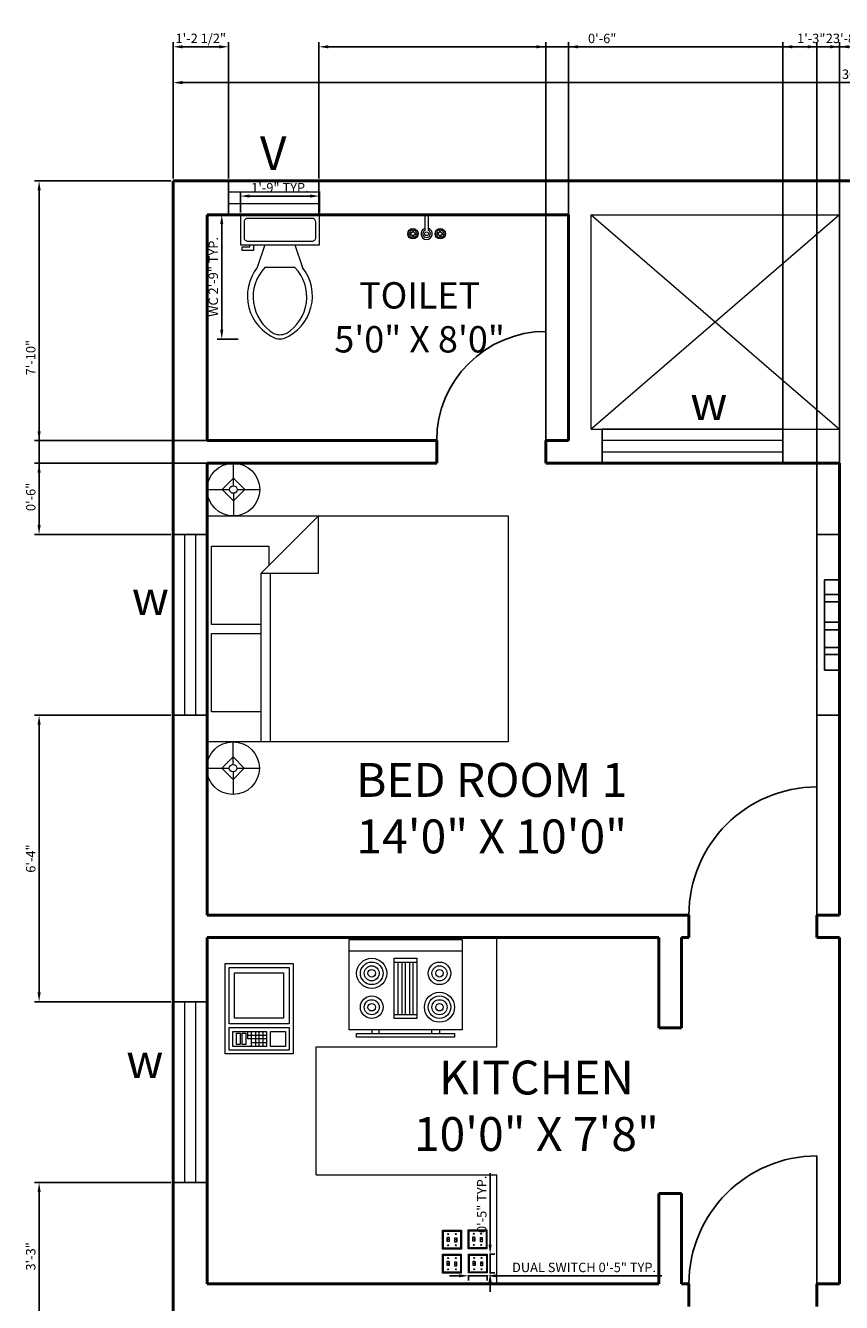
# Model space of a CAD drawing. Units: inches. Extents: x 3688 to 4628, y 1593 to 2337.
# Tile 3 of 7: x 3690 to 3907, y 1997 to 2337. Entities that reach past the tile are written whole.
import ezdxf

# ---------------------------------------------------------------- set-up
doc = ezdxf.new("R2010")
doc.units = ezdxf.units.IN
for name, color, linetype, lineweight in [('A-ANNO-DIMS', 2, 'Continuous', 18), ('A-ANNO-TEXT', 7, 'Continuous', 18), ('A-AREA-IDEN', 7, 'Continuous', 25), ('A-DOOR', 4, 'Continuous', 25), ('A-EQPM', 8, 'Continuous', 18), ('A-FLOR-FIXT', 8, 'Continuous', 18), ('A-FLOR-SHFT', 8, 'Continuous', 18), ('A-FURN', 8, 'Continuous', 18), ('A-GLAZ', 4, 'Continuous', 25), ('A-WALL', 7, 'Continuous', 50), ('E-LITE', 6, 'Continuous', 18)]:
    doc.layers.add(name, color=color, linetype=linetype, lineweight=lineweight)
doc.styles.get("Standard").update_dxf_attribs({"font": 'arial.ttf'})
doc.dimstyles.new('ISO-25', dxfattribs={"dimtxt": 2.5, "dimasz": 2.5, "dimexe": 1.25, "dimexo": 0.625, "dimtad": 1, "dimdec": 0, "dimlunit": 3, "dimtxsty": 'Standard', "dimcen": 2.5, "dimadec": 0, "dimazin": 0, "dimtfac": 1, "dimtdec": 0, "dimtmove": 0, "dimatfit": 3, "dimfxl": 1, "dimarcsym": 0})

# ---------------------------------------------------------------- blocks, each defined once
blk = doc.blocks.new('Toilet - top')
for p, q in [((9.5, -6), (9.5, -2)), ((-10, -8.5), (-8, -8.5)), ((-10, -9.5), (-10, -8.5)), ((-7, -9.5), (-10, -9.5)), ((-8, -8.5), (-8, -8)), ((-7, -8), (-7, -9.5)), ((-4, -8), (-6, -14)), ((4, -8), (6, -14)), ((4, -14), (-4, -14))]:
    blk.add_line(p, q)
blk.add_lwpolyline([(10.5, -8), (10.5, 0), (-10.5, 0), (-10.5, -8)], close=True)
for points in [[(-9.5, -2), (-9.5, -6)], [(8.5, -1), (-8.5, -1)], [(-8.5, -7), (8.5, -7)]]:
    blk.add_lwpolyline(points)
for centre, radius, start, end in [((-8.62, -1.88), 0.884, 81.8699, 188.1301), ((8.62, -1.88), 0.884, 351.8699, 98.1301), ((-8.62, -6.12), 0.884, 171.8699, 278.1301), ((8.62, -6.12), 0.884, 261.8699, 8.1301), ((3.52, -21.58), 12.17, 141.4691, 247.9714), ((4.2, -21.82), 11.33, 136.3677, 238.9468), ((-3.52, -21.58), 12.17, 292.0284, 38.5307), ((-4.2, -21.82), 11.33, 301.053, 43.6321), ((0, -27.88), 4, 245.7318, 294.2682), ((0, -29), 4, 254.8605, 285.1395)]:
    blk.add_arc(centre, radius, start, end)
blk = doc.blocks.new('Bed - Queen')
for p, q in [((0, -80.00003), (0, 0)), ((0, 0), (59.99999, 0)), ((59.99999, 0), (59.99999, -80.00003)), ((7.99999, -1.2), (28.79998, -1.2)), ((7.99999, -14.4), (7.99999, -1.2)), ((28.79998, -1.2), (28.79998, -14.4)), ((31.19999, -1.2), (51.99999, -1.2)), ((31.19999, -14.4), (31.19999, -1.2)), ((51.99999, -1.2), (51.99999, -16.4)), ((0, -14.4), (44.8, -14.4)), ((44.8, -16.8), (0, -16.8)), ((59.99999, -29.6), (44.8, -14.4)), ((44.8, -14.4), (44.8, -29.6)), ((51.99999, -16.4), (46.79936, -16.4)), ((44.8, -29.6), (59.99999, -29.6)), ((59.99999, -80.00003), (0, -80.00003))]:
    blk.add_line(p, q)
blk = doc.blocks.new('Lamp - Table')
for p, q in [((0, 7), (0, 1)), ((-1, 0), (-7, 0)), ((0, 3), (-3, 0)), ((-3, 0), (0, -3)), ((3, 0), (0, 3)), ((0, -3), (3, 0)), ((1, 0), (7, 0)), ((0, -1), (0, -7))]:
    blk.add_line(p, q)
for radius in [7, 1]:
    blk.add_circle((0, 0), radius)
blk = doc.blocks.new('Range-Oven - 30 in top')
for p, q in [((0, -3), (30, -3)), ((12, -6), (18, -6)), ((13, -20), (13, -6)), ((14, -6), (14, -20)), ((15, -20), (15, -6)), ((16, -6), (16, -20)), ((17, -20), (17, -6)), ((18, -20), (12, -20)), ((6, -24), (6, -25)), ((8, -25), (8, -24)), ((22, -25), (22, -24)), ((24, -24), (24, -25))]:
    blk.add_line(p, q)
for points in [[(0, -24), (0, 0), (30, 0), (30, -24)], [(12, -21), (12, -5), (18, -5), (18, -21)], [(2, -26), (2, -25), (28, -25), (28, -26)]]:
    blk.add_lwpolyline(points, close=True)
for centre, radius in [((6, -9), 4), ((6, -9), 3), ((24, -9), 3), ((6, -9), 2), ((6, -9), 1), ((24, -9), 2), ((24, -9), 1), ((6, -18), 3), ((6, -18), 2), ((24, -18), 4), ((24, -18), 3), ((24, -18), 2), ((6, -18), 1), ((24, -18), 1)]:
    blk.add_circle(centre, radius)
blk = doc.blocks.new('Microwave')
for p, q in [((19, 7), (19, 11)), ((20, 11), (20, 7)), ((21, 7), (21, 11)), ((18, 10), (22, 10)), ((22, 9), (18, 9)), ((18, 8), (22, 8)), ((22, 7), (18, 7)), ((19, 6), (19, 7)), ((20, 7), (20, 6)), ((20, 6), (18, 6))]:
    blk.add_line(p, q)
for points in [[(0, 0), (0, 18), (24, 18), (24, 0)], [(1, 1), (1, 17), (16, 17), (16, 1)], [(17, 1), (17, 17), (23, 17), (23, 1)], [(2.5, 2.5), (2.5, 15.5), (14.5, 15.5), (14.5, 2.5)], [(18, 12), (18, 16), (22, 16), (22, 12)], [(18, 2), (18, 11), (22, 11), (22, 2)], [(18.5, 4.5), (18.5, 5.5), (21.5, 5.5), (21.5, 4.5)], [(18.5, 3), (18.5, 4), (21.5, 4), (21.5, 3)]]:
    blk.add_lwpolyline(points, close=True)
blk = doc.blocks.new('Light Switch - Dual')
for p, q in [((-2.25, 4.75), (-2.5, 5)), ((-2.25, 4.75), (2.25, 4.75)), ((-2.25, 0.25), (-2.25, 4.75)), ((-0.875, 4), (-1.125, 4)), ((0.875, 4), (1.125, 4)), ((2.25, 4.75), (2.5, 5)), ((2.25, 4.75), (2.25, 0.25)), ((-2.25, 0.25), (-2.5, 0)), ((2.25, 0.25), (-2.25, 0.25)), ((-0.7854, 2.5), (-1.2183, 2.5)), ((-0.875, 1), (-1.125, 1)), ((0.7854, 2.5), (1.2182, 2.5)), ((0.875, 1), (1.125, 1)), ((2.25, 0.25), (2.5, 0))]:
    blk.add_line(p, q)
for points in [[(-2.5, 0), (-2.5, 5), (2.5, 5), (2.5, 0)], [(-0.78, 3.125), (-0.78, 2), (-1.22, 2), (-1.22, 3.125)], [(0.78, 1.875), (0.78, 3), (1.22, 3), (1.22, 1.875)]]:
    blk.add_lwpolyline(points, close=True)
for points in [[(-0.7818, 3), (-0.75, 3), (-0.75, 2), (-1.25, 2), (-1.25, 3), (-1.2219, 3)], [(0.7817, 2), (0.75, 2), (0.75, 3), (1.25, 3), (1.25, 2), (1.2219, 2)]]:
    blk.add_lwpolyline(points)
for centre in [(-1, 4), (1, 4), (-1, 1), (1, 1)]:
    blk.add_circle(centre, 0.125)
blk = doc.blocks.new('Faucet - Bathroom top')
for p, q in [((-4.107, 0.125), (-4.375, 0.125)), ((-3.75, 0.4788), (-3.75, 0.75)), ((-3.5, 0.482), (-3.5, 0.75)), ((-3.1461, 0.125), (-2.875, 0.125)), ((3.143, 0.125), (2.875, 0.125)), ((3.5, 0.4788), (3.5, 0.75)), ((3.75, 0.482), (3.75, 0.75)), ((4.1039, 0.125), (4.375, 0.125)), ((-4.1039, -0.125), (-4.375, -0.125)), ((-3.75, -0.4821), (-3.75, -0.75)), ((-3.5, -0.4789), (-3.5, -0.75)), ((-3.143, -0.125), (-2.875, -0.125)), ((-0.5, -0.8639), (-0.5, -4.5)), ((0.5, -4.5), (0.5, -0.8631)), ((3.1461, -0.125), (2.875, -0.125)), ((3.5, -0.4821), (3.5, -0.75)), ((3.75, -0.4789), (3.75, -0.75)), ((4.107, -0.125), (4.375, -0.125))]:
    blk.add_line(p, q)
for centre, radius in [((-3.625, 0), 1.375), ((-4.625, 0), 0.2795), ((-3.625, 0), 0.5), ((-3.625, 1), 0.2795), ((-2.625, 0), 0.2795), ((0, 0), 0.5), ((3.625, 0), 1.375), ((2.625, 0), 0.2795), ((3.625, 0), 0.5), ((3.625, 1), 0.2795), ((4.625, 0), 0.2795), ((-3.625, -1), 0.2795), ((3.625, -1), 0.2795)]:
    blk.add_circle(centre, radius)
for centre, radius, start, end in [((-3.625, 0), 1, 105.2407, 164.2093), ((-3.625, 0), 1, 16.44125, 74.07887), ((0, 0), 1.5, 289.6514, 250.3603), ((0, 0), 1, 300.3431, 239.7554), ((3.625, 0), 1, 106.12, 164.0884), ((3.625, 0), 1, 16.23422, 73.90469), ((-3.625, 0), 1, 196.2342, 253.9047), ((-3.625, 0), 1, 286.12, 344.0884), ((3.625, 0), 1, 196.4413, 254.0789), ((3.625, 0), 1, 285.2407, 344.2093), ((0, -4.5), 0.5, 180, 0)]:
    blk.add_arc(centre, radius, start, end)
blk = doc.blocks.new('*D16')
at = {"layer": 'A-ANNO-DIMS', "color": 0, "lineweight": -2, "transparency": 16777216}
for p, q in [((3729.62, 2295.94), (3729.62, 2322.66)), ((3732.12, 2321.41), (4087.12, 2321.41)), ((4089.62, 2295.94), (4089.62, 2322.66))]:
    blk.add_line(p, q, dxfattribs=at)
at = {"layer": 'A-ANNO-DIMS', "color": 0, "transparency": 16777216}
for points in [[(3732.12, 2321.83), (3732.12, 2320.99), (3729.62, 2321.41)], [(4087.12, 2321.83), (4087.12, 2320.99), (4089.62, 2321.41)]]:
    blk.add_solid(points, dxfattribs=at)
at = {"layer": 'Defpoints', "color": 0, "transparency": 16777216}
for p in [(4089.62, 2321.41), (3729.62, 2295.32), (4089.62, 2295.32)]:
    blk.add_point(p, dxfattribs=at)
at = {"layer": 'A-ANNO-DIMS', "color": 0, "transparency": 16777216, "insert": (3909.62, 2323.31), "char_height": 2.5, "attachment_point": 5}
blk.add_mtext("30'", dxfattribs=at)
blk = doc.blocks.new('DOOR-850')
blk.add_line((0, 0), (0, 34))
blk.add_arc((0, 0), 34, 0, 90)
blk = doc.blocks.new('DOOR-750')
blk.add_line((29, 0), (29, 29))
blk.add_arc((29, 0), 29, 90, 180)
blk = doc.blocks.new('WIN-1200')
for p, q in [((0, 48), (0, 0)), ((9, 48), (0, 48)), ((9, 0), (9, 48)), ((0, 0), (9, 0))]:
    blk.add_line(p, q)
blk = doc.blocks.new('WIN-600')
for p, q in [((24, 9), (0, 9)), ((0, 9), (0, 0)), ((24, 0), (24, 9)), ((0, 0), (24, 0))]:
    blk.add_line(p, q)
blk = doc.blocks.new('*D37')
at = {"layer": 'A-ANNO-DIMS', "color": 0, "lineweight": -2, "transparency": 16777216}
for p, q in [((3746.86, 2286.32), (3741.28, 2286.32)), ((3742.53, 2255.77), (3742.53, 2283.82)), ((3746.86, 2253.27), (3741.28, 2253.27))]:
    blk.add_line(p, q, dxfattribs=at)
at = {"layer": 'A-ANNO-DIMS', "color": 0, "transparency": 16777216}
for points in [[(3742.11, 2283.82), (3742.94, 2283.82), (3742.53, 2286.32)], [(3742.11, 2255.77), (3742.94, 2255.77), (3742.53, 2253.27)]]:
    blk.add_solid(points, dxfattribs=at)
at = {"layer": 'Defpoints', "color": 0, "transparency": 16777216}
for p in [(3742.53, 2286.32), (3747.48, 2286.32), (3747.48, 2253.27)]:
    blk.add_point(p, dxfattribs=at)
at = {"layer": 'A-ANNO-DIMS', "color": 0, "transparency": 16777216, "insert": (3740.61, 2269.8), "char_height": 2.5, "attachment_point": 5, "rotation": 90}
blk.add_mtext('WC 2\'-9" TYP.', dxfattribs=at)
blk = doc.blocks.new('*D38')
at = {"layer": 'A-ANNO-DIMS', "color": 0, "lineweight": -2, "transparency": 16777216}
for p, q in [((3747.48, 2286.94), (3747.48, 2292.53)), ((3749.98, 2291.28), (3765.98, 2291.28)), ((3768.48, 2286.94), (3768.48, 2292.53))]:
    blk.add_line(p, q, dxfattribs=at)
at = {"layer": 'A-ANNO-DIMS', "color": 0, "transparency": 16777216}
for points in [[(3749.98, 2291.69), (3749.98, 2290.86), (3747.48, 2291.28)], [(3765.98, 2291.69), (3765.98, 2290.86), (3768.48, 2291.28)]]:
    blk.add_solid(points, dxfattribs=at)
at = {"layer": 'Defpoints', "color": 0, "transparency": 16777216}
for p in [(3768.48, 2291.28), (3747.48, 2286.32), (3768.48, 2286.32)]:
    blk.add_point(p, dxfattribs=at)
at = {"layer": 'A-ANNO-DIMS', "color": 0, "transparency": 16777216, "insert": (3757.98, 2293.18), "char_height": 2.5, "attachment_point": 5}
blk.add_mtext('1\'-9" TYP.', dxfattribs=at)
blk = doc.blocks.new('*D49')
at = {"layer": 'A-ANNO-DIMS', "color": 0, "lineweight": -2, "transparency": 16777216}
for p, q in [((3805.56, 2004.49), (3803.06, 2004.49)), ((3808.06, 2004.61), (3808.06, 2003.24)), ((3808.06, 2004.49), (3813.06, 2004.49)), ((3813.06, 2004.61), (3813.06, 2003.24)), ((3815.56, 2004.49), (3859.45, 2004.49))]:
    blk.add_line(p, q, dxfattribs=at)
at = {"layer": 'A-ANNO-DIMS', "color": 0, "transparency": 16777216}
for points in [[(3805.56, 2004.9), (3805.56, 2004.07), (3808.06, 2004.49)], [(3815.56, 2004.9), (3815.56, 2004.07), (3813.06, 2004.49)]]:
    blk.add_solid(points, dxfattribs=at)
at = {"layer": 'Defpoints', "color": 0, "transparency": 16777216}
for p in [(3808.06, 2005.24), (3813.06, 2005.24), (3813.06, 2004.49)]:
    blk.add_point(p, dxfattribs=at)
at = {"layer": 'A-ANNO-DIMS', "color": 0, "transparency": 16777216, "insert": (3838.75, 2006.4), "char_height": 2.5, "attachment_point": 5}
blk.add_mtext('DUAL SWITCH 0\'-5" TYP.', dxfattribs=at)
blk = doc.blocks.new('*D50')
at = {"layer": 'A-ANNO-DIMS', "color": 0, "lineweight": -2, "transparency": 16777216}
for p, q in [((3813.81, 2012.74), (3813.81, 2031.73)), ((3813.68, 2010.24), (3815.06, 2010.24)), ((3813.81, 2005.24), (3813.81, 2010.24)), ((3813.68, 2005.24), (3815.06, 2005.24)), ((3813.81, 2002.74), (3813.81, 2000.24))]:
    blk.add_line(p, q, dxfattribs=at)
at = {"layer": 'A-ANNO-DIMS', "color": 0, "transparency": 16777216}
for points in [[(3813.39, 2012.74), (3814.22, 2012.74), (3813.81, 2010.24)], [(3813.39, 2002.74), (3814.22, 2002.74), (3813.81, 2005.24)]]:
    blk.add_solid(points, dxfattribs=at)
at = {"layer": 'Defpoints', "color": 0, "transparency": 16777216}
for p in [(3813.06, 2010.24), (3813.81, 2010.24), (3813.06, 2005.24)]:
    blk.add_point(p, dxfattribs=at)
at = {"layer": 'A-ANNO-DIMS', "color": 0, "transparency": 16777216, "insert": (3811.91, 2023.48), "char_height": 2.5, "attachment_point": 5, "rotation": 90}
blk.add_mtext('0\'-5" TYP.', dxfattribs=at)
blk = doc.blocks.new('*D51')
at = {"layer": 'A-ANNO-DIMS', "color": 0, "lineweight": -2, "transparency": 16777216}
for p, q in [((3729, 2295.32), (3692.77, 2295.32)), ((3694.02, 2292.82), (3694.02, 2203.89)), ((3729, 2201.39), (3692.77, 2201.39))]:
    blk.add_line(p, q, dxfattribs=at)
at = {"layer": 'A-ANNO-DIMS', "color": 0, "transparency": 16777216}
for points in [[(3693.61, 2292.82), (3694.44, 2292.82), (3694.02, 2295.32)], [(3693.61, 2203.89), (3694.44, 2203.89), (3694.02, 2201.39)]]:
    blk.add_solid(points, dxfattribs=at)
at = {"layer": 'Defpoints', "color": 0, "transparency": 16777216}
for p in [(3729.62, 2295.32), (3694.02, 2201.39), (3729.62, 2201.39)]:
    blk.add_point(p, dxfattribs=at)
at = {"layer": 'A-ANNO-DIMS', "color": 0, "transparency": 16777216, "insert": (3692.12, 2248.35), "char_height": 2.5, "attachment_point": 5, "rotation": 90}
blk.add_mtext('7\'-10"', dxfattribs=at)
blk = doc.blocks.new('*D52')
at = {"layer": 'A-ANNO-DIMS', "color": 0, "lineweight": -2, "transparency": 16777216}
for p, q in [((3729, 2153.39), (3692.77, 2153.39)), ((3694.02, 2150.89), (3694.02, 2079.76)), ((3729, 2077.26), (3692.77, 2077.26))]:
    blk.add_line(p, q, dxfattribs=at)
at = {"layer": 'A-ANNO-DIMS', "color": 0, "transparency": 16777216}
for points in [[(3693.61, 2150.89), (3694.44, 2150.89), (3694.02, 2153.39)], [(3693.61, 2079.76), (3694.44, 2079.76), (3694.02, 2077.26)]]:
    blk.add_solid(points, dxfattribs=at)
at = {"layer": 'Defpoints', "color": 0, "transparency": 16777216}
for p in [(3729.62, 2153.39), (3694.02, 2077.26), (3729.62, 2077.26)]:
    blk.add_point(p, dxfattribs=at)
at = {"layer": 'A-ANNO-DIMS', "color": 0, "transparency": 16777216, "insert": (3692.12, 2115.32), "char_height": 2.5, "attachment_point": 5, "rotation": 90}
blk.add_mtext('6\'-4"', dxfattribs=at)
blk = doc.blocks.new('*D53')
at = {"layer": 'A-ANNO-DIMS', "color": 0, "lineweight": -2, "transparency": 16777216}
for p, q in [((3729, 2029.26), (3692.77, 2029.26)), ((3694.02, 2026.76), (3694.02, 1992.54)), ((3729, 1990.04), (3692.77, 1990.04))]:
    blk.add_line(p, q, dxfattribs=at)
at = {"layer": 'A-ANNO-DIMS', "color": 0, "transparency": 16777216}
for points in [[(3693.61, 2026.76), (3694.44, 2026.76), (3694.02, 2029.26)], [(3693.61, 1992.54), (3694.44, 1992.54), (3694.02, 1990.04)]]:
    blk.add_solid(points, dxfattribs=at)
at = {"layer": 'Defpoints', "color": 0, "transparency": 16777216}
for p in [(3729.62, 2029.26), (3694.02, 1990.04), (3729.62, 1990.04)]:
    blk.add_point(p, dxfattribs=at)
at = {"layer": 'A-ANNO-DIMS', "color": 0, "transparency": 16777216, "insert": (3692.12, 2009.65), "char_height": 2.5, "attachment_point": 5, "rotation": 90}
blk.add_mtext('3\'-3"', dxfattribs=at)
blk = doc.blocks.new('*D62')
at = {"layer": 'A-ANNO-DIMS', "color": 0, "lineweight": -2, "transparency": 16777216}
for p, q in [((3729.62, 2295.94), (3729.62, 2332.17)), ((3732.12, 2330.92), (3741.8, 2330.92)), ((3744.3, 2295.94), (3744.3, 2332.17))]:
    blk.add_line(p, q, dxfattribs=at)
at = {"layer": 'A-ANNO-DIMS', "color": 0, "transparency": 16777216}
for points in [[(3732.12, 2331.34), (3732.12, 2330.5), (3729.62, 2330.92)], [(3741.8, 2331.34), (3741.8, 2330.5), (3744.3, 2330.92)]]:
    blk.add_solid(points, dxfattribs=at)
at = {"layer": 'Defpoints', "color": 0, "transparency": 16777216}
for p in [(3744.3, 2330.92), (3729.62, 2295.32), (3744.3, 2295.32)]:
    blk.add_point(p, dxfattribs=at)
at = {"layer": 'A-ANNO-DIMS', "color": 0, "transparency": 16777216, "insert": (3736.96, 2332.84), "char_height": 2.5, "attachment_point": 5}
blk.add_mtext('1\'-2 1/2"', dxfattribs=at)
blk = doc.blocks.new('*D63')
at = {"layer": 'A-ANNO-DIMS', "color": 0, "lineweight": -2, "transparency": 16777216}
for p, q in [((3768.3, 2295.94), (3768.3, 2332.17)), ((3770.8, 2330.92), (4050.42, 2330.92)), ((4052.92, 2295.94), (4052.92, 2332.17))]:
    blk.add_line(p, q, dxfattribs=at)
at = {"layer": 'A-ANNO-DIMS', "color": 0, "transparency": 16777216}
for points in [[(3770.8, 2331.34), (3770.8, 2330.5), (3768.3, 2330.92)], [(4050.42, 2331.34), (4050.42, 2330.5), (4052.92, 2330.92)]]:
    blk.add_solid(points, dxfattribs=at)
at = {"layer": 'Defpoints', "color": 0, "transparency": 16777216}
for p in [(4052.92, 2330.92), (3768.3, 2295.32), (4052.92, 2295.32)]:
    blk.add_point(p, dxfattribs=at)
at = {"layer": 'A-ANNO-DIMS', "color": 0, "transparency": 16777216, "insert": (3910.61, 2332.84), "char_height": 2.5, "attachment_point": 5}
blk.add_mtext('23\'-8 1/2"', dxfattribs=at)
blk = doc.blocks.new('*D65')
at = {"layer": 'A-ANNO-DIMS', "color": 0, "lineweight": -2, "transparency": 16777216}
for p, q in [((3891.58, 2220.94), (3891.58, 2332.17)), ((3894.08, 2330.92), (3904.12, 2330.92)), ((3906.62, 2220.94), (3906.62, 2332.17))]:
    blk.add_line(p, q, dxfattribs=at)
at = {"layer": 'A-ANNO-DIMS', "color": 0, "transparency": 16777216}
for points in [[(3894.08, 2331.34), (3894.08, 2330.5), (3891.58, 2330.92)], [(3904.12, 2331.34), (3904.12, 2330.5), (3906.62, 2330.92)]]:
    blk.add_solid(points, dxfattribs=at)
at = {"layer": 'Defpoints', "color": 0, "transparency": 16777216}
for p in [(3906.62, 2330.92), (3891.58, 2220.32), (3906.62, 2220.32)]:
    blk.add_point(p, dxfattribs=at)
at = {"layer": 'A-ANNO-DIMS', "color": 0, "transparency": 16777216, "insert": (3899.1, 2332.82), "char_height": 2.5, "attachment_point": 5}
blk.add_mtext('1\'-3"', dxfattribs=at)
blk = doc.blocks.new('*D67')
at = {"layer": 'A-ANNO-DIMS', "color": 0, "lineweight": -2, "transparency": 16777216}
for p, q in [((3826.12, 2330.92), (3823.62, 2330.92)), ((3828.62, 2226.94), (3828.62, 2332.17)), ((3828.62, 2330.92), (3834.62, 2330.92)), ((3834.62, 2226.94), (3834.62, 2332.17)), ((3837.12, 2330.92), (3847.52, 2330.92))]:
    blk.add_line(p, q, dxfattribs=at)
at = {"layer": 'A-ANNO-DIMS', "color": 0, "transparency": 16777216}
for points in [[(3826.12, 2331.34), (3826.12, 2330.5), (3828.62, 2330.92)], [(3837.12, 2331.34), (3837.12, 2330.5), (3834.62, 2330.92)]]:
    blk.add_solid(points, dxfattribs=at)
at = {"layer": 'Defpoints', "color": 0, "transparency": 16777216}
for p in [(3834.62, 2330.92), (3828.62, 2226.32), (3834.62, 2226.32)]:
    blk.add_point(p, dxfattribs=at)
at = {"layer": 'A-ANNO-DIMS', "color": 0, "transparency": 16777216, "insert": (3843.57, 2332.82), "char_height": 2.5, "attachment_point": 5}
blk.add_mtext('0\'-6"', dxfattribs=at)
blk = doc.blocks.new('*D69')
at = {"layer": 'A-ANNO-DIMS', "color": 0, "lineweight": -2, "transparency": 16777216}
for p, q in [((3694.02, 2228.82), (3694.02, 2231.32)), ((3799, 2226.32), (3692.77, 2226.32)), ((3694.02, 2226.32), (3694.02, 2220.32)), ((3799, 2220.32), (3692.77, 2220.32)), ((3694.02, 2217.82), (3694.02, 2207.42))]:
    blk.add_line(p, q, dxfattribs=at)
at = {"layer": 'A-ANNO-DIMS', "color": 0, "transparency": 16777216}
for points in [[(3693.61, 2228.82), (3694.44, 2228.82), (3694.02, 2226.32)], [(3693.61, 2217.82), (3694.44, 2217.82), (3694.02, 2220.32)]]:
    blk.add_solid(points, dxfattribs=at)
at = {"layer": 'Defpoints', "color": 0, "transparency": 16777216}
for p in [(3799.62, 2226.32), (3694.02, 2220.32), (3799.62, 2220.32)]:
    blk.add_point(p, dxfattribs=at)
at = {"layer": 'A-ANNO-DIMS', "color": 0, "transparency": 16777216, "insert": (3692.12, 2211.37), "char_height": 2.5, "attachment_point": 5, "rotation": 90}
blk.add_mtext('0\'-6"', dxfattribs=at)
blk = doc.blocks.new('*D70')
at = {"layer": 'A-ANNO-DIMS', "color": 0, "lineweight": -2, "transparency": 16777216}
for p, q in [((3898.12, 2330.92), (3895.62, 2330.92)), ((3900.62, 2100.94), (3900.62, 2332.17)), ((3900.62, 2330.92), (3906.62, 2330.92)), ((3906.62, 2100.94), (3906.62, 2332.17)), ((3909.12, 2330.92), (3919.52, 2330.92))]:
    blk.add_line(p, q, dxfattribs=at)
at = {"layer": 'A-ANNO-DIMS', "color": 0, "transparency": 16777216}
for points in [[(3898.12, 2331.34), (3898.12, 2330.5), (3900.62, 2330.92)], [(3909.12, 2331.34), (3909.12, 2330.5), (3906.62, 2330.92)]]:
    blk.add_solid(points, dxfattribs=at)
at = {"layer": 'Defpoints', "color": 0, "transparency": 16777216}
for p in [(3906.62, 2330.92), (3900.62, 2100.32), (3906.62, 2100.32)]:
    blk.add_point(p, dxfattribs=at)
at = {"layer": 'A-ANNO-DIMS', "color": 0, "transparency": 16777216, "insert": (3915.57, 2332.82), "char_height": 2.5, "attachment_point": 5}
blk.add_mtext('0\'-6"', dxfattribs=at)

msp = doc.modelspace()

# ---------------------------------------------------------------- linework, layer by layer
at = {"layer": 'A-FLOR-FIXT'}
for p, q in [((3815.62, 2065.32), (3815.62, 2094.32)), ((3732.62, 2077.26), (3732.62, 2029.26)), ((3735.62, 2029.26), (3735.62, 2077.26)), ((3767.62, 2031.32), (3767.62, 2065.32)), ((3767.62, 2065.32), (3815.62, 2065.32)), ((3900.62, 2036.32), (3900.62, 2027.42)), ((3767.62, 2031.32), (3815.62, 2031.32)), ((3815.62, 2002.32), (3815.62, 2031.32))]:
    msp.add_line(p, q, dxfattribs=at)
at = {"layer": 'A-FLOR-SHFT'}
for p, q in [((3840.62, 2229.32), (3840.62, 2286.32)), ((3840.62, 2286.32), (3906.62, 2286.32)), ((3840.62, 2286.32), (3906.62, 2229.32)), ((3906.62, 2286.32), (3840.62, 2229.32)), ((3906.62, 2229.32), (3906.62, 2286.32)), ((3906.62, 2229.32), (3906.62, 2286.32)), ((3840.62, 2229.32), (3906.62, 2229.32)), ((3891.58, 2226.32), (3843.58, 2226.32)), ((3843.58, 2223.32), (3891.58, 2223.32))]:
    msp.add_line(p, q, dxfattribs=at)
at = {"layer": 'A-FURN'}
for p, q in [((3768.3, 2292.32), (3744.3, 2292.32)), ((3744.3, 2289.32), (3768.3, 2289.32)), ((3732.62, 2201.39), (3732.62, 2153.39)), ((3735.62, 2153.39), (3735.62, 2201.39))]:
    msp.add_line(p, q, dxfattribs=at)
at = {"layer": 'A-GLAZ'}
for p, q in [((3906.62, 2201.38), (3900.62, 2201.38)), ((3900.62, 2201.38), (3900.62, 2153.38)), ((3906.62, 2201.38), (3906.62, 2189.38)), ((3906.62, 2189.38), (3902.62, 2189.38)), ((3902.62, 2189.38), (3902.62, 2165.38)), ((3906.62, 2185.46), (3902.62, 2185.46)), ((3906.62, 2183.53), (3902.62, 2183.53)), ((3906.62, 2178.08), (3902.62, 2178.08)), ((3906.62, 2176.06), (3902.62, 2176.06)), ((3906.62, 2171.38), (3902.62, 2171.38)), ((3906.62, 2169.49), (3902.62, 2169.49)), ((3902.62, 2165.38), (3906.62, 2165.38)), ((3900.62, 2153.38), (3906.62, 2153.38)), ((3906.62, 2153.38), (3906.62, 2153.38))]:
    msp.add_line(p, q, dxfattribs=at)
at = {"layer": 'A-WALL'}
for p, q in [((3729.62, 2295.32), (4089.62, 2295.32)), ((3729.62, 1695.32), (3729.62, 2295.32)), ((3738.62, 2286.32), (3834.62, 2286.32)), ((3738.62, 2226.32), (3738.62, 2286.32)), ((3834.62, 2226.32), (3834.62, 2286.32)), ((3738.62, 2226.32), (3799.62, 2226.32)), ((3799.62, 2220.32), (3799.62, 2226.32)), ((3834.62, 2226.32), (3828.62, 2226.32)), ((3828.62, 2226.32), (3828.62, 2220.32)), ((3828.62, 2226.32), (3834.62, 2226.32)), ((3738.62, 2220.32), (3799.62, 2220.32)), ((3738.62, 2100.32), (3738.62, 2220.32)), ((3828.62, 2220.32), (3906.62, 2220.32)), ((3906.62, 2100.32), (3906.62, 2220.32)), ((3738.62, 2100.32), (3866.62, 2100.32)), ((3866.62, 2100.32), (3866.62, 2094.32)), ((3900.62, 2094.32), (3900.62, 2100.32)), ((3900.62, 2094.32), (3900.62, 2100.32)), ((3900.62, 2100.32), (3906.62, 2100.32)), ((3738.62, 2094.32), (3858.62, 2094.32)), ((3738.62, 2002.32), (3738.62, 2094.32)), ((3858.62, 2094.32), (3858.62, 2070.32)), ((3858.62, 2070.32), (3858.62, 2094.32)), ((3864.62, 2094.32), (3866.62, 2094.32)), ((3864.62, 2070.32), (3864.62, 2094.32)), ((3906.62, 2094.32), (3900.62, 2094.32)), ((3900.62, 2094.32), (3906.62, 2094.32)), ((3906.62, 2094.32), (3906.62, 2002.32)), ((3858.62, 2070.32), (3864.62, 2070.32)), ((3858.62, 2002.32), (3858.62, 2026.32)), ((3858.62, 2002.32), (3858.62, 2026.32)), ((3858.62, 2026.32), (3864.62, 2026.32)), ((3864.62, 2002.32), (3864.62, 2026.32)), ((3864.62, 2026.32), (3864.62, 2002.32)), ((3738.62, 2002.32), (3858.62, 2002.32)), ((3864.62, 2002.32), (3866.62, 2002.32)), ((3866.62, 1996.32), (3866.62, 2002.32)), ((3906.62, 2002.32), (3900.62, 2002.32)), ((3900.62, 2002.32), (3900.62, 1996.32)), ((3900.62, 2002.32), (3906.62, 2002.32))]:
    msp.add_line(p, q, dxfattribs=at)

# ---------------------------------------------------------------- block references
at = {"layer": 'A-DOOR'}
msp.add_blockref('DOOR-750', (3799.62, 2226.32), dxfattribs=at)
at = {"layer": 'A-DOOR', "extrusion": (0, 0, -1), "zscale": -1}
for p in [(-3900.62, 2100.32), (-3900.62, 2002.32)]:
    msp.add_blockref('DOOR-850', p, dxfattribs=at)
at = {"layer": 'A-EQPM'}
msp.add_blockref('Range-Oven - 30 in top', (3776.36, 2093.83), dxfattribs=at)
at = {"layer": 'A-EQPM', "rotation": 270}
msp.add_blockref('Microwave', (3743.46, 2087.42), dxfattribs=at)
at = {"layer": 'A-FLOR-FIXT'}
msp.add_blockref('Toilet - top', (3757.98, 2286.32), dxfattribs=at)
at = {"layer": 'A-FLOR-FIXT', "rotation": 180}
msp.add_blockref('Faucet - Bathroom top', (3796.94, 2281.26), dxfattribs=at)
at = {"layer": 'A-FURN', "rotation": 90}
for name, p in [('Lamp - Table', (3745.62, 2213.32)), ('Bed - Queen', (3738.62, 2146.32)), ('Lamp - Table', (3745.52, 2139.32))]:
    msp.add_blockref(name, p, dxfattribs=at)
at = {"layer": 'A-GLAZ'}
for name, p in [('WIN-600', (3744.3, 2286.32)), ('WIN-1200', (3729.62, 2153.39)), ('WIN-1200', (3729.62, 2029.26))]:
    msp.add_blockref(name, p, dxfattribs=at)
at = {"layer": 'A-GLAZ', "rotation": 270}
msp.add_blockref('WIN-1200', (3843.58, 2229.32), dxfattribs=at)
at = {"layer": 'E-LITE'}
for p in [(3803.68, 2011.59), (3810.47, 2011.68), (3803.66, 2005.21), (3810.56, 2005.24)]:
    msp.add_blockref('Light Switch - Dual', p, dxfattribs=at)

# ---------------------------------------------------------------- texts
at = {"layer": 'A-ANNO-TEXT', "char_height": 9, "attachment_point": 1}
for s, heights, insert in [('\\pxqc;V', [37.18], (3686.97, 2307.16)), ('\\pxqc;w', [0], (3802.66, 2240.76)), ('\\pxqc;w', [0], (3654.34, 2189.04)), ('\\pxqc;w', [0], (3652.86, 2066.07))]:
    msp.add_mtext_dynamic_manual_height_columns(s, width=138.4723, gutter_width=12.5, heights=heights, dxfattribs=dict(at, insert=insert))
at = {"layer": 'A-AREA-IDEN', "attachment_point": 1}
for s, width, insert, char_height in [('\\pxqc;TOILET \\P5\'0" X 8\'0"', 61.3205, (3764.42, 2268.4), 7), ('\\pxqc;BED ROOM 1\\P14\'0" X 10\'0"', 105.0766, (3761.7, 2140.7), 9), ('\\pxqc;KITCHEN^J10\'0" X 7\'8"', 105.0766, (3773.56, 2061.65), 9)]:
    msp.add_mtext_dynamic_manual_height_columns(s, width=width, gutter_width=12.5, heights=[0], dxfattribs=dict(at, insert=insert, char_height=char_height))

# ---------------------------------------------------------------- dimensions: what is measured, and where the dimension line sits
at = {"layer": 'A-ANNO-DIMS'}
for base, p1, p2, override, picture, middle in [((3744.3, 2330.92), (3729.62, 2295.32), (3744.3, 2295.32), {"dimdec": 1, "dimlfac": 1, "dimrnd": 0, "dimzin": 1, "dimdsep": 46, "dimlunit": 4, "dimfrac": 2}, '*D62', (3736.96, 2332.84)), ((4052.92, 2330.92), (3768.3, 2295.32), (4052.92, 2295.32), {"dimdec": 1, "dimlfac": 1, "dimrnd": 0, "dimzin": 1, "dimdsep": 46, "dimlunit": 4, "dimfrac": 2}, '*D63', (3910.61, 2332.84)), ((3834.62, 2330.92), (3828.62, 2226.32), (3834.62, 2226.32), {"dimdec": 1, "dimlfac": 1, "dimrnd": 0, "dimzin": 1, "dimdsep": 46, "dimlunit": 4, "dimfrac": 2}, '*D67', (3843.57, 2332.82)), ((3906.62, 2330.92), (3891.58, 2220.32), (3906.62, 2220.32), {"dimdec": 1, "dimlfac": 1, "dimrnd": 0, "dimzin": 1, "dimdsep": 46, "dimlunit": 4, "dimfrac": 2}, '*D65', (3899.1, 2332.82)), ((3906.62, 2330.92), (3900.62, 2100.32), (3906.62, 2100.32), {"dimdec": 1, "dimlfac": 1, "dimrnd": 0, "dimzin": 1, "dimdsep": 46, "dimlunit": 4, "dimfrac": 2}, '*D70', (3915.57, 2332.82)), ((4089.62, 2321.41), (3729.62, 2295.32), (4089.62, 2295.32), {"dimclrd": 0, "dimclre": 0, "dimclrt": 0}, '*D16', (3909.62, 2323.31))]:
    dim = msp.add_linear_dim(base=base, p1=p1, p2=p2, dimstyle='ISO-25', override=override, dxfattribs=at)
    dim.commit()
    dim.dimension.update_dxf_attribs({"geometry": picture, "text_midpoint": middle})
for base, p1, p2, text, picture, middle in [((3768.48, 2291.28), (3747.48, 2286.32), (3768.48, 2286.32), '<> TYP.', '*D38', (3757.98, 2293.18)), ((3813.06, 2004.49), (3808.06, 2005.24), (3813.06, 2005.24), 'DUAL SWITCH <> TYP.', '*D49', (3838.75, 2006.4))]:
    dim = msp.add_linear_dim(base=base, p1=p1, p2=p2, text=text, dimstyle='ISO-25', override={"dimdec": 1, "dimrnd": 0, "dimzin": 1, "dimlunit": 4, "dimfrac": 2}, dxfattribs=at)
    dim.commit()
    dim.dimension.update_dxf_attribs({"geometry": picture, "text_midpoint": middle})
for base, p1, p2, picture, middle in [((3694.02, 2201.39), (3729.62, 2295.32), (3729.62, 2201.39), '*D51', (3692.12, 2248.35)), ((3694.02, 2220.32), (3799.62, 2226.32), (3799.62, 2220.32), '*D69', (3692.12, 2211.37)), ((3694.02, 2077.26), (3729.62, 2153.39), (3729.62, 2077.26), '*D52', (3692.12, 2115.32)), ((3694.02, 1990.04), (3729.62, 2029.26), (3729.62, 1990.04), '*D53', (3692.12, 2009.65))]:
    dim = msp.add_linear_dim(base=base, p1=p1, p2=p2, angle=90, dimstyle='ISO-25', override={"dimdec": 1, "dimlfac": 1, "dimrnd": 0, "dimzin": 1, "dimdsep": 46, "dimlunit": 4, "dimfrac": 2}, dxfattribs=at)
    dim.commit()
    dim.dimension.update_dxf_attribs({"geometry": picture, "text_midpoint": middle})
for base, p1, p2, text, picture, middle in [((3742.5266, 2286.32), (3747.4835, 2253.2737), (3747.4835, 2286.32), 'WC <> TYP.', '*D37', (3740.609, 2269.7969)), ((3813.81, 2010.24), (3813.06, 2005.24), (3813.06, 2010.24), '<> TYP.', '*D50', (3811.91, 2023.48))]:
    dim = msp.add_linear_dim(base=base, p1=p1, p2=p2, angle=90, text=text, dimstyle='ISO-25', override={"dimdec": 1, "dimrnd": 0, "dimzin": 1, "dimlunit": 4, "dimfrac": 2}, dxfattribs=at)
    dim.commit()
    dim.dimension.update_dxf_attribs({"geometry": picture, "text_midpoint": middle})

doc.saveas('drawing.dxf')
